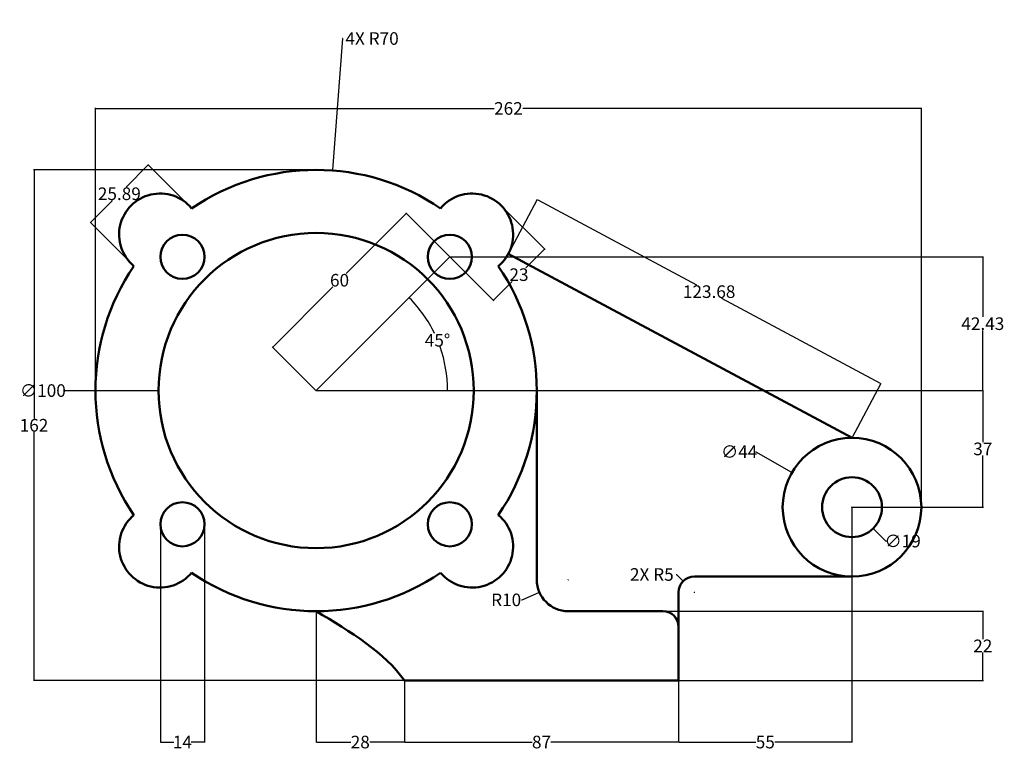
# Model space of a CAD drawing. Units: millimetres. Extents: x -69 to 244, y -102 to 129.
import ezdxf

# ---------------------------------------------------------------- set-up
doc = ezdxf.new("R2010")
doc.units = ezdxf.units.MM
doc.header["$MEASUREMENT"] = 0
for name, color, linetype, lineweight in [('M-CONS', 8, 'Continuous', 18), ('M-DIMS', 2, 'Continuous', 25), ('M-OUTL', 7, 'Continuous', 50)]:
    doc.layers.add(name, color=color, linetype=linetype, lineweight=lineweight)
doc.styles.get("Standard").update_dxf_attribs({"font": 'arial.ttf'})
doc.dimstyles.get("Standard").update_dxf_attribs({"dimtxt": 4, "dimasz": 0.18, "dimexe": 0.18, "dimexo": 0.0625, "dimgap": 0.09, "dimtad": 0, "dimtih": 1, "dimtoh": 1, "dimdec": 1, "dimzin": 0, "dimdsep": 46, "dimtxsty": 'Standard', "dimcen": 0.09, "dimclrd": 3, "dimclre": 3, "dimclrt": 1, "dimadec": 0, "dimazin": 0, "dimtfac": 1, "dimtdec": 1, "dimtofl": 0, "dimtmove": 0, "dimatfit": 3, "dimfxl": 1, "dimtolj": 1, "dimtzin": 0, "dimlwd": -1, "dimlwe": -1, "dimarcsym": 0})

# ---------------------------------------------------------------- blocks, each defined once
blk = doc.blocks.new('*U1')
blk.add_circle((-6.54, -6.54), 7)
blk.add_arc((0.54, 0.54), 13, 309.672, 140.328)
blk = doc.blocks.new('*U2')
at = {"layer": 'M-OUTL', "color": 0, "linetype": 'ByBlock', "lineweight": -2, "transparency": 16777216}
for p, rotation in [((-23.59, 60.76), 90.00000000000003), ((-23.59, -37.17), 180), ((74.33, -37.17), 270)]:
    blk.add_blockref('*U1', p, dxfattribs=dict(at, rotation=rotation))
blk.add_blockref('*U1', (74.33, 60.76), dxfattribs=at)
blk = doc.blocks.new('*D3')
at = {"layer": 'Defpoints', "color": 0, "transparency": 16777216}
for p in [(67.8, 54.22), (65.65, 22.58), (25.37, 11.79), (25.37, 11.79), (75.37, 11.79)]:
    blk.add_point(p, dxfattribs=at)
at = {"layer": 'M-DIMS', "color": 0, "transparency": 16777216}
for start, end in [(25.6979, 44.7527), (0.2473, 19.3744)]:
    blk.add_arc((25.37, 11.79), 41.7, start, end, dxfattribs=at)
for points in [[(54.96, 41.13), (55, 41.17), (54.86, 41.28)], [(67.1, 11.97), (67.04, 11.97), (67.07, 11.79)]]:
    blk.add_solid(points, dxfattribs=at)
at = {"layer": 'M-DIMS', "color": 0, "transparency": 16777216, "insert": (63.89, 27.75), "char_height": 4, "attachment_point": 5}
blk.add_mtext('\\A1;45°', dxfattribs=at)
blk = doc.blocks.new('*D4')
at = {"layer": 'Defpoints', "color": 0, "transparency": 16777216}
for p in [(217.37, 101.29), (-44.63, 11.79), (217.37, -25.21)]:
    blk.add_point(p, dxfattribs=at)
at = {"layer": 'M-DIMS', "color": 3, "transparency": 16777216}
for p, q in [((-44.63, 11.86), (-44.63, 101.47)), ((-44.45, 101.29), (81.85, 101.29)), ((217.19, 101.29), (90.9, 101.29)), ((217.37, -25.14), (217.37, 101.47))]:
    blk.add_line(p, q, dxfattribs=at)
for points in [[(-44.45, 101.32), (-44.45, 101.26), (-44.63, 101.29)], [(217.19, 101.32), (217.19, 101.26), (217.37, 101.29)]]:
    blk.add_solid(points, dxfattribs=at)
at = {"layer": 'M-DIMS', "color": 1, "transparency": 16777216, "insert": (86.37, 101.29), "char_height": 4, "attachment_point": 5}
blk.add_mtext('\\A1;262', dxfattribs=at)
blk = doc.blocks.new('*D5')
at = {"layer": 'Defpoints', "color": 0, "transparency": 16777216}
for p in [(25.37, 81.79), (-64.13, -80.21), (53.37, -80.21)]:
    blk.add_point(p, dxfattribs=at)
at = {"layer": 'M-DIMS', "color": 3, "transparency": 16777216}
for p, q in [((25.31, 81.79), (-64.31, 81.79)), ((-64.13, 81.61), (-64.13, 2.93)), ((-64.13, -80.03), (-64.13, -1.34)), ((53.31, -80.21), (-64.31, -80.21))]:
    blk.add_line(p, q, dxfattribs=at)
for points in [[(-64.16, 81.61), (-64.1, 81.61), (-64.13, 81.79)], [(-64.16, -80.03), (-64.1, -80.03), (-64.13, -80.21)]]:
    blk.add_solid(points, dxfattribs=at)
at = {"layer": 'M-DIMS', "color": 1, "transparency": 16777216, "insert": (-64.13, 0.79), "char_height": 4, "attachment_point": 5}
blk.add_mtext('\\A1;162', dxfattribs=at)
blk = doc.blocks.new('*D6')
at = {"layer": 'Defpoints', "color": 0, "transparency": 16777216}
for p in [(25.37, -58.21), (53.37, -80.21), (53.37, -99.71)]:
    blk.add_point(p, dxfattribs=at)
at = {"layer": 'M-DIMS', "color": 3, "transparency": 16777216}
for p, q in [((25.37, -58.27), (25.37, -99.89)), ((53.37, -80.27), (53.37, -99.89)), ((25.55, -99.71), (36.38, -99.71)), ((53.19, -99.71), (42.37, -99.71))]:
    blk.add_line(p, q, dxfattribs=at)
for points in [[(25.55, -99.68), (25.55, -99.74), (25.37, -99.71)], [(53.19, -99.68), (53.19, -99.74), (53.37, -99.71)]]:
    blk.add_solid(points, dxfattribs=at)
at = {"layer": 'M-DIMS', "color": 1, "transparency": 16777216, "insert": (39.37, -99.71), "char_height": 4, "attachment_point": 5}
blk.add_mtext('\\A1;28', dxfattribs=at)
blk = doc.blocks.new('*D7')
at = {"layer": 'Defpoints', "color": 0, "transparency": 16777216}
for p in [(53.37, -80.21), (140.37, -80.21), (140.37, -99.71)]:
    blk.add_point(p, dxfattribs=at)
at = {"layer": 'M-DIMS', "color": 3, "transparency": 16777216}
for p, q in [((53.37, -80.27), (53.37, -99.89)), ((140.37, -80.27), (140.37, -99.89)), ((53.55, -99.71), (93.92, -99.71)), ((140.19, -99.71), (99.83, -99.71))]:
    blk.add_line(p, q, dxfattribs=at)
for points in [[(53.55, -99.68), (53.55, -99.74), (53.37, -99.71)], [(140.19, -99.68), (140.19, -99.74), (140.37, -99.71)]]:
    blk.add_solid(points, dxfattribs=at)
at = {"layer": 'M-DIMS', "color": 1, "transparency": 16777216, "insert": (96.87, -99.71), "char_height": 4, "attachment_point": 5}
blk.add_mtext('\\A1;87', dxfattribs=at)
blk = doc.blocks.new('*D8')
at = {"layer": 'Defpoints', "color": 0, "transparency": 16777216}
for p in [(195.37, -25.21), (140.37, -80.21), (195.37, -99.71)]:
    blk.add_point(p, dxfattribs=at)
at = {"layer": 'M-DIMS', "color": 3, "transparency": 16777216}
for p, q in [((195.37, -25.27), (195.37, -99.89)), ((140.37, -80.27), (140.37, -99.89)), ((140.55, -99.71), (164.9, -99.71)), ((195.19, -99.71), (170.84, -99.71))]:
    blk.add_line(p, q, dxfattribs=at)
for points in [[(140.55, -99.68), (140.55, -99.74), (140.37, -99.71)], [(195.19, -99.68), (195.19, -99.74), (195.37, -99.71)]]:
    blk.add_solid(points, dxfattribs=at)
at = {"layer": 'M-DIMS', "color": 1, "transparency": 16777216, "insert": (167.87, -99.71), "char_height": 4, "attachment_point": 5}
blk.add_mtext('\\A1;55', dxfattribs=at)
blk = doc.blocks.new('*D9')
at = {"layer": 'Defpoints', "color": 0, "transparency": 16777216}
for p in [(25.37, 11.79), (195.37, -25.21), (236.87, -25.21)]:
    blk.add_point(p, dxfattribs=at)
at = {"layer": 'M-DIMS', "color": 3, "transparency": 16777216}
for p, q in [((25.44, 11.79), (237.05, 11.79)), ((236.87, 11.61), (236.87, -4.57)), ((236.87, -25.03), (236.87, -8.84)), ((195.44, -25.21), (237.05, -25.21))]:
    blk.add_line(p, q, dxfattribs=at)
for points in [[(236.84, 11.61), (236.9, 11.61), (236.87, 11.79)], [(236.84, -25.03), (236.9, -25.03), (236.87, -25.21)]]:
    blk.add_solid(points, dxfattribs=at)
at = {"layer": 'M-DIMS', "color": 1, "transparency": 16777216, "insert": (236.87, -6.71), "char_height": 4, "attachment_point": 5}
blk.add_mtext('\\A1;37', dxfattribs=at)
blk = doc.blocks.new('*D10')
at = {"layer": 'Defpoints', "color": 0, "transparency": 16777216}
for p in [(54.01, 68.01), (67.8, 54.22), (25.37, 11.79)]:
    blk.add_point(p, dxfattribs=at)
at = {"layer": 'M-DIMS', "color": 3, "transparency": 16777216}
for p, q in [((53.88, 67.88), (34.93, 48.93)), ((67.75, 54.26), (53.88, 68.14)), ((11.71, 25.71), (30.67, 44.66)), ((25.33, 11.84), (11.46, 25.71))]:
    blk.add_line(p, q, dxfattribs=at)
for points in [[(53.86, 67.9), (53.9, 67.86), (54.01, 68.01)], [(11.69, 25.73), (11.73, 25.69), (11.58, 25.58)]]:
    blk.add_solid(points, dxfattribs=at)
at = {"layer": 'M-DIMS', "color": 1, "transparency": 16777216, "insert": (32.8, 46.79), "char_height": 4, "attachment_point": 5}
blk.add_mtext('\\A1;60', dxfattribs=at)
blk = doc.blocks.new('*D11')
at = {"layer": 'Defpoints', "color": 0, "transparency": 16777216}
for p in [(135.37, -58.21), (140.37, -80.21), (236.87, -80.21)]:
    blk.add_point(p, dxfattribs=at)
at = {"layer": 'M-DIMS', "color": 3, "transparency": 16777216}
for p, q in [((135.44, -58.21), (237.05, -58.21)), ((236.87, -58.39), (236.87, -67.11)), ((236.87, -80.03), (236.87, -71.31)), ((140.44, -80.21), (237.05, -80.21))]:
    blk.add_line(p, q, dxfattribs=at)
for points in [[(236.84, -58.39), (236.9, -58.39), (236.87, -58.21)], [(236.84, -80.03), (236.9, -80.03), (236.87, -80.21)]]:
    blk.add_solid(points, dxfattribs=at)
at = {"layer": 'M-DIMS', "color": 1, "transparency": 16777216, "insert": (236.87, -69.21), "char_height": 4, "attachment_point": 5}
blk.add_mtext('\\A1;22', dxfattribs=at)
blk = doc.blocks.new('*D12')
at = {"layer": 'Defpoints', "color": 0, "transparency": 16777216}
for p in [(-24.05, -30.63), (-10.05, -30.63), (-10.05, -99.71)]:
    blk.add_point(p, dxfattribs=at)
at = {"layer": 'M-DIMS', "color": 3, "transparency": 16777216}
for p, q in [((-24.05, -30.7), (-24.05, -99.89)), ((-10.05, -30.7), (-10.05, -99.89)), ((-23.87, -99.71), (-19.81, -99.71)), ((-10.23, -99.71), (-14.3, -99.71))]:
    blk.add_line(p, q, dxfattribs=at)
for points in [[(-23.87, -99.68), (-23.87, -99.74), (-24.05, -99.71)], [(-10.23, -99.68), (-10.23, -99.74), (-10.05, -99.71)]]:
    blk.add_solid(points, dxfattribs=at)
at = {"layer": 'M-DIMS', "color": 1, "transparency": 16777216, "insert": (-17.05, -99.71), "char_height": 4, "attachment_point": 5}
blk.add_mtext('\\A1;14', dxfattribs=at)
blk = doc.blocks.new('*D13')
at = {"layer": 'Defpoints', "color": 0, "transparency": 16777216}
for p in [(-27.91, 83.38), (-14.12, 69.59), (-32.42, 51.28)]:
    blk.add_point(p, dxfattribs=at)
at = {"layer": 'M-DIMS', "color": 3, "transparency": 16777216}
for p, q in [((-28.03, 83.25), (-34.93, 76.36)), ((-14.16, 69.63), (-28.03, 83.51)), ((-46.09, 65.2), (-39.19, 72.09)), ((-32.47, 51.33), (-46.34, 65.2))]:
    blk.add_line(p, q, dxfattribs=at)
for points in [[(-28.06, 83.27), (-28.01, 83.23), (-27.91, 83.38)], [(-46.11, 65.22), (-46.06, 65.18), (-46.21, 65.07)]]:
    blk.add_solid(points, dxfattribs=at)
at = {"layer": 'M-DIMS', "color": 1, "transparency": 16777216, "insert": (-37.06, 74.23), "char_height": 4, "attachment_point": 5}
blk.add_mtext('\\A1;25.89', dxfattribs=at)
blk = doc.blocks.new('*D14')
at = {"layer": 'Defpoints', "color": 0, "transparency": 16777216}
for p in [(67.8, 54.22), (236.87, 54.22), (25.37, 11.79)]:
    blk.add_point(p, dxfattribs=at)
at = {"layer": 'M-DIMS', "color": 3, "transparency": 16777216}
for p, q in [((67.86, 54.22), (237.05, 54.22)), ((236.87, 54.04), (236.87, 35.14)), ((236.87, 11.97), (236.87, 30.87)), ((25.44, 11.79), (237.05, 11.79))]:
    blk.add_line(p, q, dxfattribs=at)
for points in [[(236.84, 54.04), (236.9, 54.04), (236.87, 54.22)], [(236.84, 11.97), (236.9, 11.97), (236.87, 11.79)]]:
    blk.add_solid(points, dxfattribs=at)
at = {"layer": 'M-DIMS', "color": 1, "transparency": 16777216, "insert": (236.87, 33.01), "char_height": 4, "attachment_point": 5}
blk.add_mtext('\\A1;42.43', dxfattribs=at)
blk = doc.blocks.new('*D15')
at = {"layer": 'Defpoints', "color": 0, "transparency": 16777216}
for p in [(84.06, 70.48), (67.8, 54.22), (81.59, 40.43)]:
    blk.add_point(p, dxfattribs=at)
at = {"layer": 'M-DIMS', "color": 3, "transparency": 16777216}
for p, q in [((84.11, 70.44), (97.98, 56.57)), ((97.72, 56.57), (91.85, 50.7)), ((67.84, 54.18), (81.71, 40.3)), ((81.71, 40.56), (87.59, 46.43))]:
    blk.add_line(p, q, dxfattribs=at)
for points in [[(97.7, 56.59), (97.75, 56.55), (97.85, 56.69)], [(81.69, 40.58), (81.74, 40.54), (81.59, 40.43)]]:
    blk.add_solid(points, dxfattribs=at)
at = {"layer": 'M-DIMS', "color": 1, "transparency": 16777216, "insert": (89.72, 48.56), "char_height": 4, "attachment_point": 5}
blk.add_mtext('\\A1;23', dxfattribs=at)
blk = doc.blocks.new('*D16')
at = {"layer": 'Defpoints', "color": 0, "transparency": 16777216}
for p in [(86.33, 55.16), (204.57, 13.99), (195.37, -3.21)]:
    blk.add_point(p, dxfattribs=at)
at = {"layer": 'M-DIMS', "color": 3, "transparency": 16777216}
for p, q in [((86.36, 55.21), (95.62, 72.51)), ((95.69, 72.26), (146.07, 45.3)), ((204.42, 14.07), (154.04, 41.03)), ((195.4, -3.15), (204.66, 14.14))]:
    blk.add_line(p, q, dxfattribs=at)
for points in [[(95.71, 72.29), (95.68, 72.24), (95.53, 72.35)], [(204.43, 14.1), (204.4, 14.04), (204.57, 13.99)]]:
    blk.add_solid(points, dxfattribs=at)
at = {"layer": 'M-DIMS', "color": 1, "transparency": 16777216, "insert": (150.05, 43.17), "char_height": 4, "attachment_point": 5}
blk.add_mtext('\\A1;123.68', dxfattribs=at)
blk = doc.blocks.new('*D17')
at = {"layer": 'Defpoints', "color": 0, "transparency": 16777216}
for p in [(30.58, 81.6), (25.37, 11.79)]:
    blk.add_point(p, dxfattribs=at)
at = {"layer": 'M-DIMS', "color": 3, "transparency": 16777216}
for p, q in [((33.7, 123.48), (30.59, 81.78)), ((33.88, 123.48), (33.7, 123.48)), ((25.28, 11.79), (25.46, 11.79)), ((25.37, 11.7), (25.37, 11.88))]:
    blk.add_line(p, q, dxfattribs=at)
blk.add_solid([(30.56, 81.78), (30.62, 81.78), (30.58, 81.6)], dxfattribs=at)
at = {"layer": 'M-DIMS', "color": 1, "transparency": 16777216, "insert": (43.12, 123.48), "char_height": 4, "attachment_point": 5}
blk.add_mtext('\\A1;4X R70', dxfattribs=at)
blk = doc.blocks.new('*D18')
at = {"layer": 'Defpoints', "color": 0, "transparency": 16777216}
for p in [(-24.63, 11.79), (75.37, 11.79)]:
    blk.add_point(p, dxfattribs=at)
at = {"layer": 'M-DIMS', "color": 3, "transparency": 16777216}
for p, q in [((-54.63, 11.79), (-24.81, 11.79)), ((25.28, 11.79), (25.46, 11.79)), ((25.37, 11.7), (25.37, 11.88))]:
    blk.add_line(p, q, dxfattribs=at)
blk.add_solid([(-24.81, 11.82), (-24.81, 11.76), (-24.63, 11.79)], dxfattribs=at)
at = {"layer": 'M-DIMS', "color": 1, "transparency": 16777216, "insert": (-61.31, 11.79), "char_height": 4, "attachment_point": 5}
blk.add_mtext('\\A1;∅100', dxfattribs=at)
blk = doc.blocks.new('*D19')
at = {"layer": 'Defpoints', "color": 0, "transparency": 16777216}
for p in [(176.32, -14.21), (214.43, -36.21)]:
    blk.add_point(p, dxfattribs=at)
at = {"layer": 'M-DIMS', "color": 3, "transparency": 16777216}
for p, q in [((164.71, -7.61), (164.89, -7.61)), ((164.89, -7.61), (176.16, -14.12)), ((195.28, -25.21), (195.46, -25.21)), ((195.37, -25.3), (195.37, -25.12))]:
    blk.add_line(p, q, dxfattribs=at)
blk.add_solid([(176.18, -14.09), (176.15, -14.14), (176.32, -14.21)], dxfattribs=at)
at = {"layer": 'M-DIMS', "color": 1, "transparency": 16777216, "insert": (159.59, -7.61), "char_height": 4, "attachment_point": 5}
blk.add_mtext('\\A1;∅44', dxfattribs=at)
blk = doc.blocks.new('*D20')
at = {"layer": 'Defpoints', "color": 0, "transparency": 16777216}
for p in [(188.66, -18.49), (202.09, -31.92)]:
    blk.add_point(p, dxfattribs=at)
at = {"layer": 'M-DIMS', "color": 3, "transparency": 16777216}
for p, q in [((195.28, -25.21), (195.46, -25.21)), ((195.37, -25.3), (195.37, -25.12)), ((206.12, -35.95), (202.22, -32.05)), ((206.3, -35.95), (206.12, -35.95))]:
    blk.add_line(p, q, dxfattribs=at)
blk.add_solid([(202.24, -32.03), (202.2, -32.07), (202.09, -31.92)], dxfattribs=at)
at = {"layer": 'M-DIMS', "color": 1, "transparency": 16777216, "insert": (211.44, -35.95), "char_height": 4, "attachment_point": 5}
blk.add_mtext('\\A1;∅19', dxfattribs=at)
blk = doc.blocks.new('*D21')
at = {"layer": 'Defpoints', "color": 0, "transparency": 16777216}
for p in [(105.37, -48.21), (96.21, -52.2)]:
    blk.add_point(p, dxfattribs=at)
at = {"layer": 'M-DIMS', "color": 3, "transparency": 16777216}
for p, q in [((105.28, -48.21), (105.46, -48.21)), ((105.37, -48.3), (105.37, -48.12)), ((90.71, -54.6), (96.04, -52.27)), ((90.53, -54.6), (90.71, -54.6))]:
    blk.add_line(p, q, dxfattribs=at)
blk.add_solid([(96.03, -52.25), (96.05, -52.3), (96.21, -52.2)], dxfattribs=at)
at = {"layer": 'M-DIMS', "color": 1, "transparency": 16777216, "insert": (85.66, -54.6), "char_height": 4, "attachment_point": 5}
blk.add_mtext('\\A1;R10', dxfattribs=at)
blk = doc.blocks.new('*D22')
at = {"layer": 'Defpoints', "color": 0, "transparency": 16777216}
for p in [(141.84, -48.67), (145.37, -52.21)]:
    blk.add_point(p, dxfattribs=at)
at = {"layer": 'M-DIMS', "color": 3, "transparency": 16777216}
for p, q in [((139.54, -46.55), (139.72, -46.55)), ((139.72, -46.55), (141.71, -48.54)), ((145.28, -52.21), (145.46, -52.21)), ((145.37, -52.3), (145.37, -52.12))]:
    blk.add_line(p, q, dxfattribs=at)
blk.add_solid([(141.73, -48.52), (141.69, -48.57), (141.84, -48.67)], dxfattribs=at)
at = {"layer": 'M-DIMS', "color": 1, "transparency": 16777216, "insert": (131.87, -46.55), "char_height": 4, "attachment_point": 5}
blk.add_mtext('\\A1;2X R5', dxfattribs=at)

msp = doc.modelspace()

# ---------------------------------------------------------------- linework, layer by layer
at = {"layer": 'M-CONS'}
for q in [(67.799, 54.22), (75.373, 11.793)]:
    msp.add_line((25.373, 11.793), q, dxfattribs=at)
at = {"layer": 'M-OUTL'}
for p, q in [((195.373, -3.207), (86.332, 55.156)), ((86.332, 55.156), (86.332, 55.156)), ((95.373, 11.793), (95.373, -48.207)), ((195.373, -47.207), (145.373, -47.207)), ((195.373, -47.207), (145.373, -47.207)), ((140.373, -52.207), (140.373, -80.207)), ((105.373, -58.207), (135.373, -58.207)), ((130.373, -58.207), (125.373, -58.207)), ((135.373, -58.207), (130.373, -58.207)), ((135.373, -58.207), (135.373, -58.207)), ((140.373, -63.207), (140.373, -80.207)), ((53.373, -80.207), (140.373, -80.207))]:
    msp.add_line(p, q, dxfattribs=at)
for centre, radius in [((25.373, 11.793), 50), ((195.373, -25.207), 22), ((195.373, -25.207), 9.5)]:
    msp.add_circle(centre, radius, dxfattribs=at)
for centre, radius, start, end in [((25.373, 11.793), 70, 55.656, 124.344), ((25.373, 11.793), 70, 145.656, 214.344), ((25.373, 11.793), 70, 325.656, 34.344), ((25.373, 11.793), 70, 235.656, 304.344), ((105.373, -48.207), 10, 180, 270), ((145.373, -52.207), 5, 90, 180), ((135.373, -63.207), 5, 0, 90)]:
    msp.add_arc(centre, radius, start, end, dxfattribs=at)
msp.add_open_spline([(25.373, -58.207), (36.31, -64.761), (47.248, -71.314), (53.373, -80.207)], degree=3, dxfattribs=at)

# ---------------------------------------------------------------- block references
msp.add_blockref('*U2', (0, 0), dxfattribs=at)

# ---------------------------------------------------------------- dimensions: what is measured, and where the dimension line sits
at = {"layer": 'M-DIMS'}
for center, mpoint, text, picture, middle in [((25.373, 11.793), (30.578, 81.599), '4X <>', '*D17', (43.121, 123.483)), ((145.373, -52.207), (141.837, -48.671), '2X <>', '*D22', (131.874, -46.55))]:
    dim = msp.add_radius_dim(center=center, mpoint=mpoint, text=text, dimstyle='Standard', override={"dimdec": 0, "dimlfac": 1, "dimrnd": 0, "dimzin": 0, "dimdsep": 46, "dimlunit": 2}, dxfattribs=at)
    dim.commit()
    dim.dimension.update_dxf_attribs({"geometry": picture, "text_midpoint": middle, "dimtype": 164})
for base, p1, p2, picture, middle in [((217.373, 101.293), (-44.627, 11.793), (217.373, -25.207), '*D4', (86.373, 101.293)), ((195.373, -99.707), (140.373, -80.207), (195.373, -25.207), '*D8', (167.873, -99.707)), ((-10.054, -99.707), (-24.054, -30.633), (-10.054, -30.633), '*D12', (-17.054, -99.707)), ((53.373, -99.707), (25.373, -58.207), (53.373, -80.207), '*D6', (39.373, -99.707)), ((140.373, -99.707), (53.373, -80.207), (140.373, -80.207), '*D7', (96.873, -99.707))]:
    dim = msp.add_linear_dim(base=base, p1=p1, p2=p2, dimstyle='Standard', override={"dimdec": 0, "dimlfac": 1, "dimrnd": 0, "dimzin": 0, "dimdsep": 46, "dimlunit": 2}, dxfattribs=at)
    dim.commit()
    dim.dimension.update_dxf_attribs({"geometry": picture, "text_midpoint": middle})
for base, p1, p2, angle, override, picture, middle in [((-64.127, -80.207), (25.373, 81.793), (53.373, -80.207), 90, {"dimdec": 0, "dimlfac": 1, "dimrnd": 0, "dimzin": 0, "dimdsep": 46, "dimlunit": 2}, '*D5', (-64.127, 0.793)), ((-27.907, 83.378), (-32.424, 51.284), (-14.119, 69.59), 45, {"dimdec": 2, "dimlfac": 1, "dimrnd": 0, "dimzin": 0, "dimdsep": 46, "dimlunit": 2}, '*D13', (-37.06, 74.226)), ((204.575, 13.985), (86.332, 55.156), (195.373, -3.207), 331.84264, {"dimdec": 2, "dimlfac": 1, "dimrnd": 0, "dimzin": 0, "dimdsep": 46, "dimlunit": 2}, '*D16', (150.054, 43.167)), ((81.588, 40.431), (84.063, 70.483), (67.799, 54.22), 225, {"dimdec": 0, "dimlfac": 1, "dimrnd": 0, "dimzin": 0, "dimdsep": 46, "dimlunit": 2}, '*D15', (89.719, 48.563)), ((54.011, 68.008), (25.373, 11.793), (67.799, 54.22), 45, {"dimdec": 0, "dimlfac": 1, "dimrnd": 0, "dimzin": 0, "dimdsep": 46, "dimlunit": 2}, '*D10', (32.797, 46.795)), ((236.873, 54.22), (25.373, 11.793), (67.799, 54.22), 90, {"dimdec": 2, "dimlfac": 1, "dimrnd": 0, "dimzin": 0, "dimdsep": 46, "dimlunit": 2}, '*D14', (236.873, 33.006)), ((236.873, -25.207), (25.373, 11.793), (195.373, -25.207), 90, {"dimdec": 0, "dimlfac": 1, "dimrnd": 0, "dimzin": 0, "dimdsep": 46, "dimlunit": 2}, '*D9', (236.873, -6.707)), ((236.873, -80.207), (135.373, -58.207), (140.373, -80.207), 90, {"dimdec": 0, "dimlfac": 1, "dimrnd": 0, "dimzin": 0, "dimdsep": 46, "dimlunit": 2}, '*D11', (236.873, -69.207))]:
    dim = msp.add_linear_dim(base=base, p1=p1, p2=p2, angle=angle, dimstyle='Standard', override=override, dxfattribs=at)
    dim.commit()
    dim.dimension.update_dxf_attribs({"geometry": picture, "text_midpoint": middle})
dim = msp.add_angular_dim_2l(base=(65.648, 22.585), line1=((25.373, 11.793), (67.799, 54.22)), line2=((25.373, 11.793), (75.373, 11.793)), dimstyle='Standard', override={"dimclrd": 0, "dimclre": 0, "dimclrt": 0}, dxfattribs=at)
dim.commit()
dim.dimension.update_dxf_attribs({"geometry": '*D3', "text_midpoint": (63.895, 27.749)})
for p1, p2, picture, middle in [((75.373, 11.793), (-24.627, 11.793), '*D18', (-54.627, 11.793)), ((214.425, -36.207), (176.32, -14.207), '*D19', (159.586, -7.607)), ((188.655, -18.489), (202.09, -31.924), '*D20', (211.436, -35.955))]:
    dim = msp.add_diameter_dim_2p(p1=p1, p2=p2, dimstyle='Standard', override={"dimdec": 0, "dimlfac": 1, "dimrnd": 0, "dimzin": 0, "dimdsep": 46, "dimlunit": 2}, dxfattribs=at)
    dim.commit()
    dim.dimension.update_dxf_attribs({"geometry": picture, "text_midpoint": middle, "dimtype": 163})
dim = msp.add_radius_dim(center=(105.373, -48.207), mpoint=(96.206, -52.203), dimstyle='Standard', override={"dimdec": 0, "dimlfac": 1, "dimrnd": 0, "dimzin": 0, "dimdsep": 46, "dimlunit": 2}, dxfattribs=at)
dim.commit()
dim.dimension.update_dxf_attribs({"geometry": '*D21', "text_midpoint": (85.664, -54.601), "dimtype": 164})

doc.saveas('drawing.dxf')
